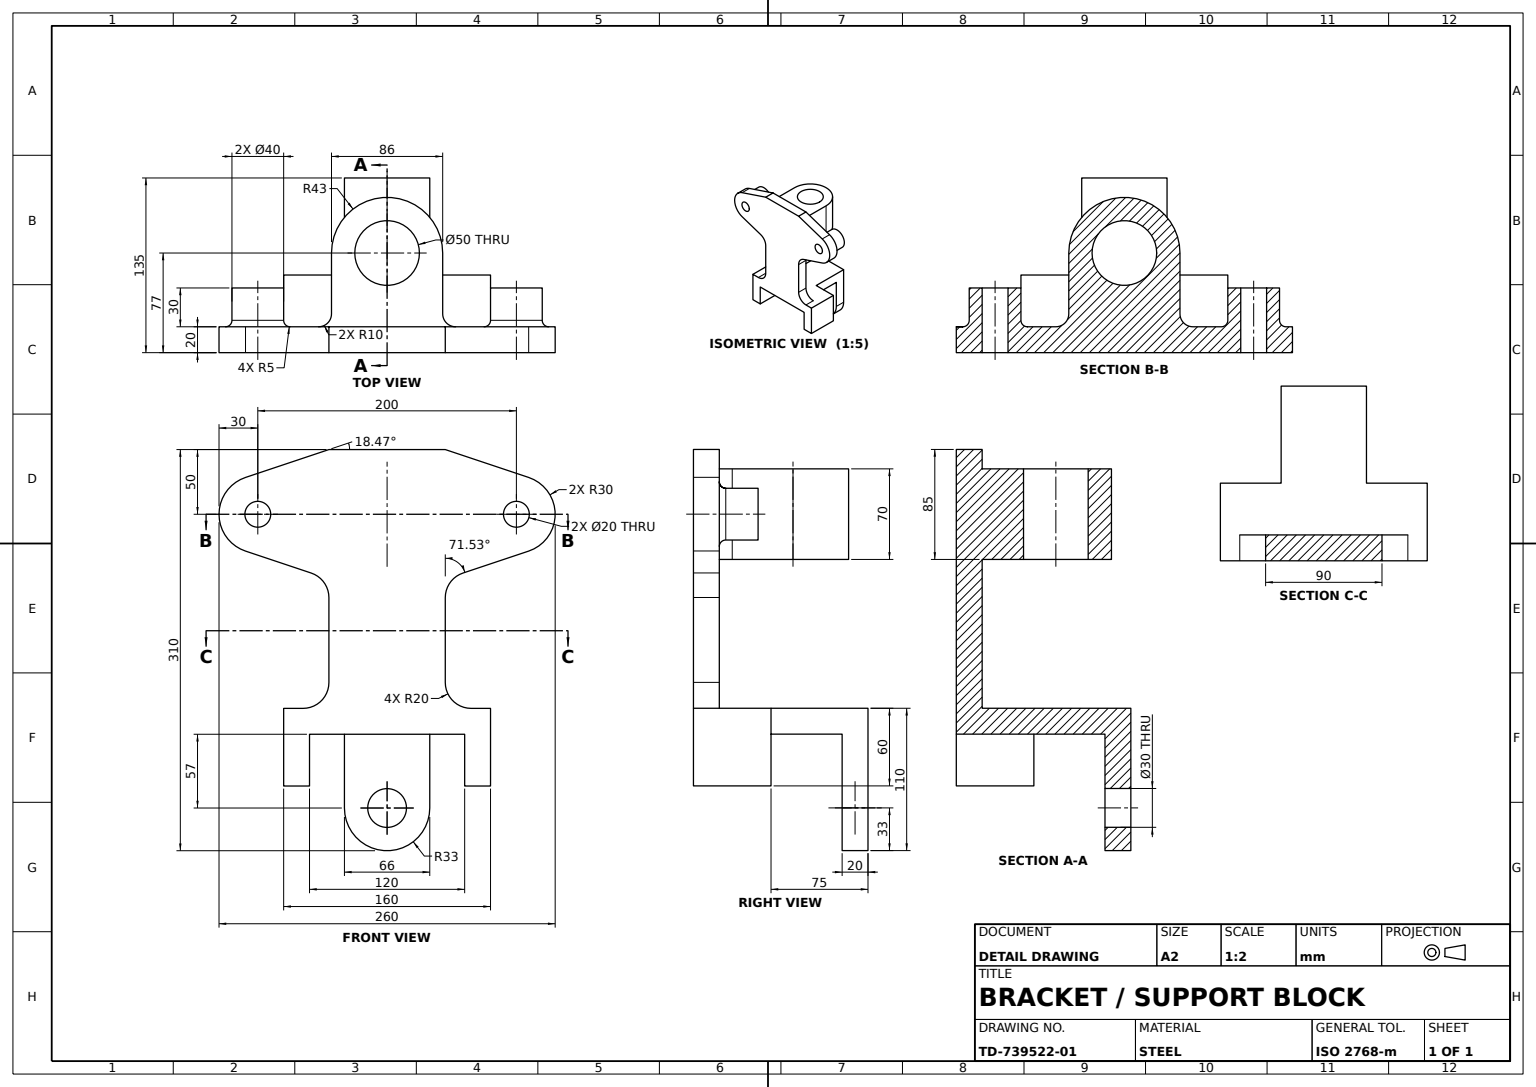
SolidWorks part; units mm, degrees
material "Plain Carbon Steel"
ref_plane "Front Plane" through (0, 0, 0) normal (0, 0, 1) x (1, 0, 0)
ref_plane "Top Plane" through (0, 0, 0) normal (0, 1, 0) x (1, 0, 0)
ref_plane "Right Plane" through (0, 0, 0) normal (1, 0, 0) x (0, 0, -1)
sketch "Base Profile Sketch" plane through (0, 0, 0) normal (1, 0, 0) x (0, 0, -1)
  line L0 (0, 0) -> (0, 33.4022) construction
  line L1 (45, 50) -> (-45, 50)
  line L2 (109.5043, 28.4547) -> (45, 50)
  line L3 (-45, 50) -> (-109.5043, 28.4547)
  line L4 (100, 0) -> (60.1283, 0) construction
  line L5 (-58.6638, -45.4361) -> (-109.5043, -28.4547)
  line L6 (109.5043, -28.4547) -> (58.6638, -45.4361)
  line L7 (-45, -64.4059) -> (-45, -150)
  line L8 (45, -64.4059) -> (45, -150)
  line L9 (45, -150) -> (-45, -150)
  arc A0 (109.5043, -28.4547) -> (109.5043, 28.4547) centre (100, 0) ccw
  arc A1 (-109.5043, 28.4547) -> (-109.5043, -28.4547) centre (-100, 0) ccw
  arc A2 (58.6638, -45.4361) -> (45, -64.4059) centre (65, -64.4059) ccw
  arc A3 (-58.6638, -45.4361) -> (-45, -64.4059) centre (-65, -64.4059) cw
  arc A4 (70, 0) -> (109.5043, -28.4547) centre (100, 0) ccw construction
  arc A5 (109.5043, 28.4547) -> (70, 0) centre (100, 0) ccw construction
  arc A6 (-109.5043, -28.4547) -> (-109.5043, 28.4547) centre (-100, 0) ccw construction
  point P11 (0, 50)
  point P21 (45, -50)
  point P24 (-45, -50)
  dimension "D1" = 30
  dimension "D6" = 20
  dimension "D2" = 200
  dimension "D3" = 90
  dimension "D4" = 50
  dimension "D5" = 100
extrude "Base Body" add sketch "Base Profile Sketch" along normal blind 20
sketch "Hub Boss Sketch" plane through (0, 0, 0) normal (-1, 0, 0) x (0, 0, 1)
  line L0 (0, 0) -> (0, 43.8312) construction
  circle A0 centre (-100, 0) radius 20
  circle A1 centre (100, 0) radius 20
  arc A2 (-109.5043, 28.4547) -> (-109.5043, -28.4547) centre (-100, 0) ccw construction
  dimension "D1" = 40
extrude "Hub Boss" add sketch "Hub Boss Sketch" along normal blind 30
sketch "Hub Bore Sketch" plane through (-30, 0, 0) normal (-1, 0, 0) x (0, 0, 1)
  circle A0 centre (-100, 0) radius 10
  circle A1 centre (100, 0) radius 10
  dimension "D1" = 20
extrude "Hub Bore Ø20" cut sketch "Hub Bore Sketch" against normal through all
sketch "Foot Block Sketch" plane through (0, 0, 0) normal (0, 1, 0) x (1, 0, 0)
  line L0 (-57, 43) -> (0, 43)
  line L1 (0, 45) -> (0, -45) construction
  line L2 (0, 43) -> (0, -43)
  line L3 (0, -43) -> (-57, -43)
  arc A0 (-57, 43) -> (-57, -43) centre (-57, 0) ccw
  arc A1 (-57, -43) -> (-57, 43) centre (-57, 0) ccw construction
  circle A2 centre (-57, 0) radius 25
  point P6 (-100, 0)
  dimension "D3" = 50
  dimension "D1" = 86
  dimension "D2" = 100
extrude "Foot Block" add sketch "Foot Block Sketch" along normal mid plane 70
sketch "Hinge Plate Sketch" plane through (0, -150, 0) normal (0, -1, 0) x (1, 0, 0)
  line L0 (20, 0) -> (20, 80)
  line L1 (20, 45) -> (20, -45) construction
  line L2 (20, 109.5043) -> (20, 58.6638) construction
  line L3 (20, 80) -> (-40, 80)
  line L4 (-40, 80) -> (-40, 33)
  line L5 (-40, 33) -> (-115, 33)
  line L6 (-115, 33) -> (-115, -33)
  line L7 (-115, -33) -> (-40, -33)
  line L8 (-40, -33) -> (-40, -80)
  line L9 (-40, -80) -> (20, -80)
  line L10 (20, -58.6638) -> (20, -109.5043) construction
  line L11 (20, -80) -> (20, 0)
  line L12 (0, 0) -> (-21.6061, 0) construction
  line L13 (0, 45) -> (0, -45) construction
  dimension "D1" = 160
  dimension "D2" = 60
  dimension "D3" = 75
  dimension "D4" = 66
extrude "Hinge Plate" add sketch "Hinge Plate Sketch" along normal blind 20
sketch "Plate Stiffener Sketch" plane through (-115, 0, 0) normal (-1, 0, 0) x (0, 0, 1)
  line L0 (33, -170) -> (33, -150) construction
  line L1 (-33, -150) -> (33, -150)
  line L2 (-33, -150) -> (-33, -227)
  line L3 (-33, -227) -> (33, -227) construction
  line L4 (33, -150) -> (33, -227)
  arc A0 (33, -227) -> (-33, -227) centre (0, -227) cw
  circle A1 centre (0, -227) radius 15
  point P8 (0, -260)
  dimension "D2" = 30
  dimension "D1" = 110
extrude "Plate Stiffener" add sketch "Plate Stiffener Sketch" against normal blind 20
sketch "Pin Boss Sketch" plane through (0, 0, 80) normal (0, 0, 1) x (1, 0, 0)
  line L0 (20, -170) -> (20, -150) construction
  line L1 (-40, -150) -> (20, -150)
  line L2 (-40, -150) -> (-40, -210)
  line L3 (-40, -210) -> (20, -210)
  line L4 (20, -150) -> (20, -210)
  line L5 (-40, -150) -> (-115, -150) construction
  dimension "D1" = 60
extrude "Pin Boss" add sketch "Pin Boss Sketch" against normal blind 20
mirror "Pin Boss Mirror" about plane through (0, 0, 0) normal (0, 0, 1) of "Pin Boss"
fillet "Hub Fillet R5" radius 5 2 edges at (0, 0, -120) (0, 0, 80)
fillet "Foot Block Fillet R10" radius 10 2 edges at (0, 0, -43) (0, 0, 43)
fillet "Hinge Plate Fillet R20" radius 20 2 edges at (10, -150, -45) (10, -150, 45)
